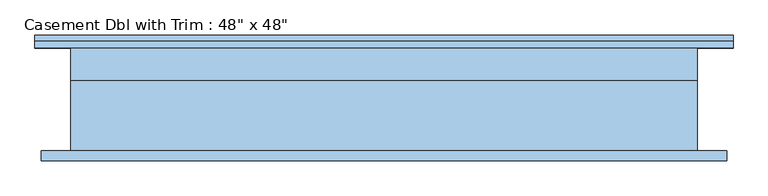
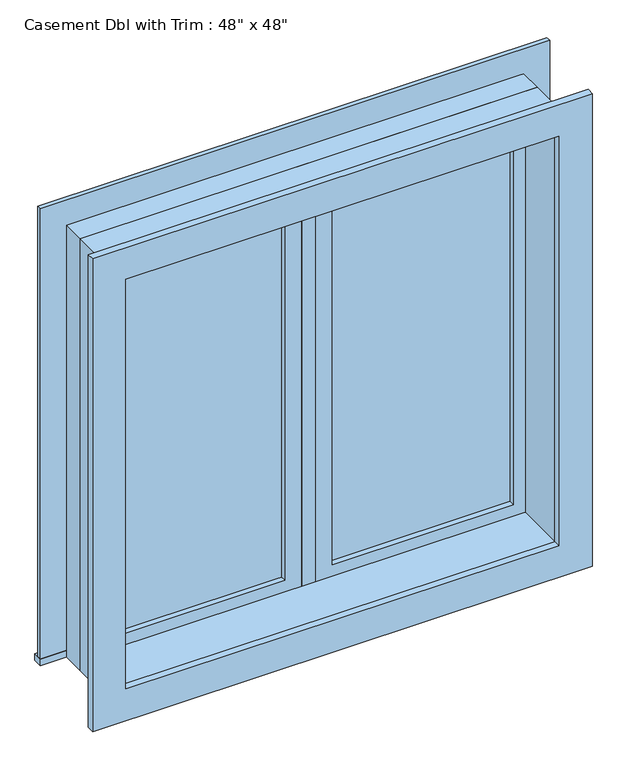
"""IFC4 building model written with IfcOpenShell, lengths in millimetres: window geometry."""

from ifc_helpers import new_model, si_unit, frame, origin, place, context, project, spatial, polyline, outline, extrude, source, transform, mapped, element, save


def window_264d1730(model_context):
    return source(origin(), model_context, "Body", "SweptSolid", [
        extrude(outline(polyline([(63.5, 84.125), (546.1, 84.125), (546.1, 71.425), (63.5, 71.425), (63.5, 84.125)])), frame((0.0, 0.0, 977.9), z_axis=(0.0, 0.0, 1.0), x_axis=(1.0, 0.0, 0.0)), (0.0, 0.0, 1.0), 1092.2),
        extrude(outline(polyline([(2114.55, 19.05), (933.45, 19.05), (933.45, 590.55), (2114.55, 590.55), (2114.55, 19.05)]), holes=[polyline([(2070.1, 63.5), (2070.1, 546.1), (977.9, 546.1), (977.9, 63.5), (2070.1, 63.5)])]), frame((0.0, 55.55, 0.0), z_axis=(0.0, 1.0, 0.0), x_axis=(0.0, 0.0, 1.0)), (0.0, 0.0, 1.0), 44.45),
        extrude(outline(polyline([(19.05, 55.55), (-19.05, 55.55), (-19.05, 119.05), (19.05, 119.05), (19.05, 55.55)])), frame((0.0, 0.0, 933.45), z_axis=(0.0, 0.0, 1.0), x_axis=(1.0, 0.0, 0.0)), (0.0, 0.0, 1.0), 1181.1),
        extrude(outline(polyline([(-679.45, 144.45), (679.45, 144.45), (679.45, 119.05), (-679.45, 119.05), (-679.45, 144.45)])), frame((0.0, 0.0, 914.4), z_axis=(0.0, 0.0, 1.0), x_axis=(1.0, 0.0, 0.0)), (0.0, 0.0, 1.0), 19.05),
        extrude(outline(polyline([(2114.55, -590.55), (2114.55, 590.55), (933.45, 590.55), (933.45, 679.45), (2203.45, 679.45), (2203.45, -679.45), (933.45, -679.45), (933.45, -590.55), (2114.55, -590.55)])), frame((0.0, 119.05, 0.0), z_axis=(0.0, 1.0, 0.0), x_axis=(0.0, 0.0, 1.0)), (0.0, 0.0, 1.0), 12.7),
        extrude(outline(polyline([(2190.75, 666.75), (2190.75, -666.75), (857.25, -666.75), (857.25, 666.75), (2190.75, 666.75)]), holes=[polyline([(2101.85, 577.85), (946.15, 577.85), (946.15, -577.85), (2101.85, -577.85), (2101.85, 577.85)])]), frame((0.0, -100.0, 0.0), z_axis=(0.0, 1.0, 0.0), x_axis=(0.0, 0.0, 1.0)), (0.0, 0.0, 1.0), 19.05),
        extrude(outline(polyline([(-63.5, 71.425), (-546.1, 71.425), (-546.1, 84.125), (-63.5, 84.125), (-63.5, 71.425)])), frame((0.0, 0.0, 977.9), z_axis=(0.0, 0.0, 1.0), x_axis=(1.0, 0.0, 0.0)), (0.0, 0.0, 1.0), 1092.2),
        extrude(outline(polyline([(2114.55, -590.55), (933.45, -590.55), (933.45, -19.05), (2114.55, -19.05), (2114.55, -590.55)]), holes=[polyline([(2070.1, -546.1), (2070.1, -63.5), (977.9, -63.5), (977.9, -546.1), (2070.1, -546.1)])]), frame((0.0, 55.55, 0.0), z_axis=(0.0, 1.0, 0.0), x_axis=(0.0, 0.0, 1.0)), (0.0, 0.0, 1.0), 44.45),
        extrude(outline(polyline([(2133.6, -609.6), (914.4, -609.6), (914.4, 609.6), (2133.6, 609.6), (2133.6, -609.6)]), holes=[polyline([(2101.85, -577.85), (2101.85, 577.85), (946.15, 577.85), (946.15, -577.85), (2101.85, -577.85)])]), frame((0.0, -80.95, 0.0), z_axis=(0.0, 1.0, 0.0), x_axis=(0.0, 0.0, 1.0)), (0.0, 0.0, 1.0), 136.5),
        extrude(outline(polyline([(2133.6, 609.6), (2133.6, -609.6), (914.4, -609.6), (914.4, 609.6), (2133.6, 609.6)]), holes=[polyline([(2114.55, 590.55), (933.45, 590.55), (933.45, -590.55), (2114.55, -590.55), (2114.55, 590.55)])]), frame((0.0, 55.55, 0.0), z_axis=(0.0, 1.0, 0.0), x_axis=(0.0, 0.0, 1.0)), (0.0, 0.0, 1.0), 63.5),
    ])


if __name__ == "__main__":
    model = new_model("IFC4")
    model_context = context("Model", 3, world=origin())
    ifc_project = project(units=[si_unit("LENGTHUNIT", "METRE", prefix="MILLI")], contexts=[model_context])
    site = spatial("IfcSite", under=ifc_project)
    building = spatial("IfcBuilding", under=site)
    placement = place(None, origin())
    window_shape = window_264d1730(model_context)
    element("IfcWindow", 1, ObjectType="Casement Dbl with Trim : 48\" x 48\"", at=placement, inside=building, context=model_context, shape_type="MappedRepresentation", body=[
        mapped(window_shape, transform((0.0, 0.0, 0.0), x_axis=(1.0, 0.0, 0.0), y_axis=(0.0, 1.0, 0.0), z_axis=(0.0, 0.0, 1.0))),
    ])
    save(model, "model.ifc")

# Revit data of these elements
# Type "Casement Dbl with Trim : 48\" x 48\""
#   Type Mark = "19"
#   Construction Type Id = "GSP4R"
#   Assembly Code = "B2020100"
#   Analytic Construction = "1/8 in Pilkington single glazing"
#   Visual Light Transmittance = 0.9
#   Solar Heat Gain Coefficient = 0.78
#   Heat Transfer Coefficient (U) = 3.6886 W/(m²·K)
#   Height = 4' - 0"
#   Default Sill Height = 3' - 0"
#   Trim Projection - Ext. = 0' - 0 1/2"
#   Trim Projection - Int. = 0' - 0 3/4"
#   Trim Width - Exterior = 0' - 3 1/2"
#   Trim Width - Interior = 0' - 3 1/2"
#   Width = 4' - 0"
#   Window Inset = 0' - 0 3/4"
#   Define Thermal Properties by = 1
#   Glass Pane Material = Glass
#   Sash Material = Sash
#   Trim Exterior Material = Trim
#   Trim Interior Material = Trim
#   Wall Closure = (empty or 0)
# Element 1 (IfcWindow, "Casement Dbl with Trim : 48\" x 48\"")
#   Materials on its faces: "Sash", "Trim", "Glass"
# Materials
#   "Glass": class "Glass", colour RGB 218 227 224, transparency 0.85, Description = "Soda Lime Glass", Cost = 0
#   "Sash": class "Wood", colour RGB 136 99 55, transparency 0
#   "Trim": class "Wood", colour RGB 224 178 126, transparency 0
